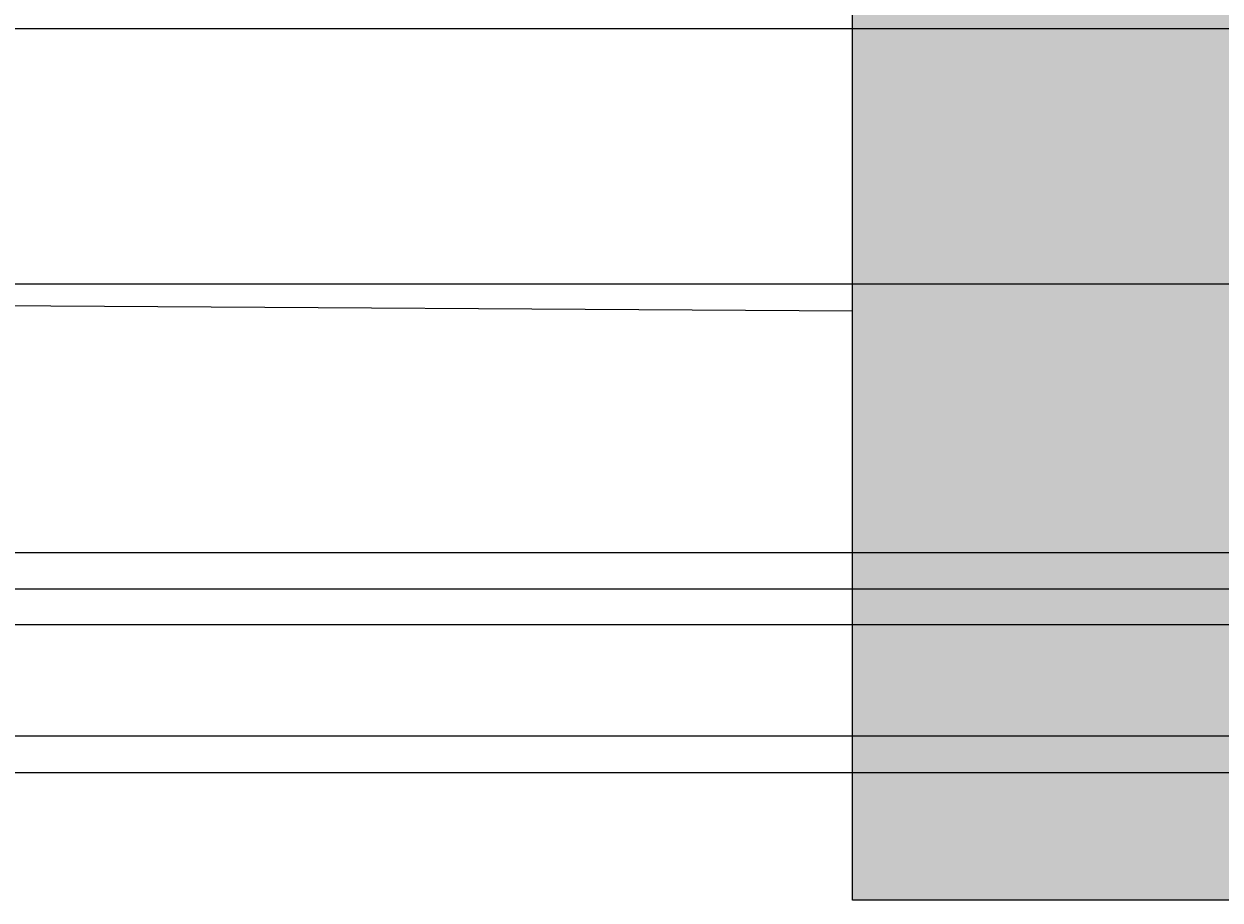
# Model space of a CAD drawing. Units: inches. Extents: x 35362 to 73946, y 43607 to 67532.
# Tile 12 of 134: x 43509 to 46225, y 46919 to 48909. Entities that reach past the tile are written whole.
import ezdxf

# ---------------------------------------------------------------- set-up
doc = ezdxf.new("R2010")
doc.units = ezdxf.units.IN
doc.header["$MEASUREMENT"] = 0
for name, color, linetype, lineweight in [('A-ANNO-DIMS', 2, 'Continuous', 18), ('E-SYMB', 1, 'Continuous', 25), ('E-SYMB-PATT', 1, 'Continuous', 13), ('E-WIRE', 3, 'Continuous', 25)]:
    doc.layers.add(name, color=color, linetype=linetype, lineweight=lineweight)
doc.styles.get("Standard").update_dxf_attribs({"font": 'arial.ttf'})
doc.dimstyles.get("Standard").update_dxf_attribs({"dimtxt": 0.18, "dimasz": 0.18, "dimexe": 0.18, "dimexo": 0.0625, "dimgap": 0.09, "dimtad": 0, "dimtih": 1, "dimtoh": 1, "dimdec": 4, "dimzin": 0, "dimdsep": 46, "dimtxsty": 'Standard', "dimcen": 0.09, "dimadec": 0, "dimazin": 0, "dimtfac": 1, "dimtdec": 4, "dimtofl": 0, "dimtmove": 0, "dimatfit": 3, "dimfxl": 1, "dimtolj": 1, "dimtzin": 0, "dimarcsym": 0})

# ---------------------------------------------------------------- blocks, each defined once
blk = doc.blocks.new('*D43')
at = {"layer": 'A-ANNO-DIMS', "color": 0, "lineweight": -2, "transparency": 16777216}
for p, q in [((62004.7, 47625.2), (35361.8, 47625.2)), ((35361.9, 47625), (35361.9, 47416.9)), ((35361.9, 47208.4), (35361.9, 47416.5)), ((62004.7, 47208.2), (35361.8, 47208.2))]:
    blk.add_line(p, q, dxfattribs=at)
at = {"layer": 'A-ANNO-DIMS', "color": 0, "transparency": 16777216}
for points in [[(35361.9, 47625), (35362, 47625), (35361.9, 47625.2)], [(35361.9, 47208.4), (35362, 47208.4), (35361.9, 47208.2)]]:
    blk.add_solid(points, dxfattribs=at)
at = {"layer": 'Defpoints', "color": 0, "transparency": 16777216}
for p in [(62004.7, 47625.2), (35361.9, 47208.2), (62004.7, 47208.2)]:
    blk.add_point(p, dxfattribs=at)
at = {"layer": 'A-ANNO-DIMS', "color": 0, "transparency": 16777216, "insert": (35361.9, 47416.7), "char_height": 0.18, "attachment_point": 5}
blk.add_mtext('\\A1;416.9', dxfattribs=at)
blk = doc.blocks.new('*D67')
at = {"layer": 'A-ANNO-DIMS', "color": 0, "lineweight": -2, "transparency": 16777216}
for p, q in [((56873.5, 53351.5), (35361.8, 53351.5)), ((35361.9, 53351.3), (35361.9, 49400.9)), ((35361.9, 45450.1), (35361.9, 49400.5)), ((53793.6, 45449.9), (35361.8, 45449.9))]:
    blk.add_line(p, q, dxfattribs=at)
at = {"layer": 'A-ANNO-DIMS', "color": 0, "transparency": 16777216}
for points in [[(35361.9, 53351.3), (35362, 53351.3), (35361.9, 53351.5)], [(35361.9, 45450.1), (35362, 45450.1), (35361.9, 45449.9)]]:
    blk.add_solid(points, dxfattribs=at)
at = {"layer": 'Defpoints', "color": 0, "transparency": 16777216}
for p in [(35361.9, 53351.5), (56873.6, 53351.5), (53793.6, 45449.9)]:
    blk.add_point(p, dxfattribs=at)
at = {"layer": 'A-ANNO-DIMS', "color": 0, "transparency": 16777216, "insert": (35361.9, 49400.7), "char_height": 0.18, "attachment_point": 5}
blk.add_mtext('\\A1;7901.6', dxfattribs=at)
blk = doc.blocks.new('*D87')
at = {"layer": 'A-ANNO-DIMS', "color": 0, "lineweight": -2, "transparency": 16777216}
for p, q in [((52362.5, 48318.3), (35361.8, 48318.3)), ((35361.9, 48318.1), (35361.9, 47931.4)), ((35361.9, 47544.3), (35361.9, 47931)), ((52362.5, 47544.1), (35361.8, 47544.1))]:
    blk.add_line(p, q, dxfattribs=at)
at = {"layer": 'A-ANNO-DIMS', "color": 0, "transparency": 16777216}
for points in [[(35361.9, 48318.1), (35362, 48318.1), (35361.9, 48318.3)], [(35361.9, 47544.3), (35362, 47544.3), (35361.9, 47544.1)]]:
    blk.add_solid(points, dxfattribs=at)
at = {"layer": 'Defpoints', "color": 0, "transparency": 16777216}
for p in [(35361.9, 48318.3), (52362.6, 48318.3), (52362.6, 47544.1)]:
    blk.add_point(p, dxfattribs=at)
at = {"layer": 'A-ANNO-DIMS', "color": 0, "transparency": 16777216, "insert": (35361.9, 47931.2), "char_height": 0.18, "attachment_point": 5}
blk.add_mtext('\\A1;774.1', dxfattribs=at)
blk = doc.blocks.new('*D89')
at = {"layer": 'A-ANNO-DIMS', "color": 0, "lineweight": -2, "transparency": 16777216}
for p, q in [((53707.7, 48897.7), (35361.8, 48897.7)), ((35361.9, 48897.6), (35361.9, 48303.2)), ((35361.9, 47708.4), (35361.9, 48302.8)), ((53707.7, 47708.2), (35361.8, 47708.2))]:
    blk.add_line(p, q, dxfattribs=at)
at = {"layer": 'A-ANNO-DIMS', "color": 0, "transparency": 16777216}
for points in [[(35361.9, 48897.6), (35362, 48897.6), (35361.9, 48897.7)], [(35361.9, 47708.4), (35362, 47708.4), (35361.9, 47708.2)]]:
    blk.add_solid(points, dxfattribs=at)
at = {"layer": 'Defpoints', "color": 0, "transparency": 16777216}
for p in [(53707.8, 48897.7), (35361.9, 47708.2), (53707.8, 47708.2)]:
    blk.add_point(p, dxfattribs=at)
at = {"layer": 'A-ANNO-DIMS', "color": 0, "transparency": 16777216, "insert": (35361.9, 48303), "char_height": 0.18, "attachment_point": 5}
blk.add_mtext('\\A1;1189.5', dxfattribs=at)
blk = doc.blocks.new('*D90')
at = {"layer": 'A-ANNO-DIMS', "color": 0, "lineweight": -2, "transparency": 16777216}
for p, q in [((53707.7, 47291.3), (35361.8, 47291.3)), ((35361.9, 47291.1), (35361.9, 46710.3)), ((35361.9, 46129.1), (35361.9, 46709.9)), ((53793.6, 46128.9), (35361.8, 46128.9))]:
    blk.add_line(p, q, dxfattribs=at)
at = {"layer": 'A-ANNO-DIMS', "color": 0, "transparency": 16777216}
for points in [[(35361.9, 47291.1), (35362, 47291.1), (35361.9, 47291.3)], [(35361.9, 46129.1), (35362, 46129.1), (35361.9, 46128.9)]]:
    blk.add_solid(points, dxfattribs=at)
at = {"layer": 'Defpoints', "color": 0, "transparency": 16777216}
for p in [(53707.8, 47291.3), (35361.9, 46128.9), (53793.6, 46128.9)]:
    blk.add_point(p, dxfattribs=at)
at = {"layer": 'A-ANNO-DIMS', "color": 0, "transparency": 16777216, "insert": (35361.9, 46710.1), "char_height": 0.18, "attachment_point": 5}
blk.add_mtext('\\A1;1162.4', dxfattribs=at)

msp = doc.modelspace()

# ---------------------------------------------------------------- hatches: boundary and pattern name
at = {"layer": 'E-SYMB-PATT'}
h = msp.add_hatch(color=256, dxfattribs=at)
h.dxf.hatch_style = 1
h.paths.add_polyline_path([(48163.038, 49689.843), (45390.147, 49689.843), (45390.147, 46919.381), (48163.038, 46919.381)])

# ---------------------------------------------------------------- linework, layer by layer
at = {"layer": 'E-SYMB'}
msp.add_lwpolyline([(45390.147, 49689.843), (48163.038, 49689.843), (48163.038, 46919.381), (45390.147, 46919.381)], close=True, dxfattribs=at)
at = {"layer": 'E-WIRE'}
msp.add_line((42373.206, 48275.646), (45390.147, 48257.489), dxfattribs=at)

# ---------------------------------------------------------------- dimensions: what is measured, and where the dimension line sits
at = {"layer": 'A-ANNO-DIMS'}
for base, p1, p2, picture, middle in [((35361.949, 53351.529), (53793.638, 45449.894), (56873.602, 53351.529), '*D67', (35361.949, 49400.712)), ((35361.949, 47708.216), (53707.781, 48897.738), (53707.781, 47708.216), '*D89', (35361.949, 48302.977)), ((35361.949, 48318.269), (52362.557, 47544.134), (52362.557, 48318.269), '*D87', (35361.949, 47931.201)), ((35361.949, 47208.25), (62004.728, 47625.181), (62004.728, 47208.25), '*D43', (35361.949, 47416.715)), ((35361.949, 46128.878), (53707.781, 47291.285), (53793.638, 46128.878), '*D90', (35361.949, 46710.081))]:
    dim = msp.add_linear_dim(base=base, p1=p1, p2=p2, angle=90, dimstyle='Standard', override={"dimdec": 1, "dimlfac": 1, "dimrnd": 0, "dimzin": 0, "dimdsep": 46, "dimlunit": 2}, dxfattribs=at)
    dim.commit()
    dim.dimension.update_dxf_attribs({"geometry": picture, "text_midpoint": middle})

doc.saveas('drawing.dxf')
